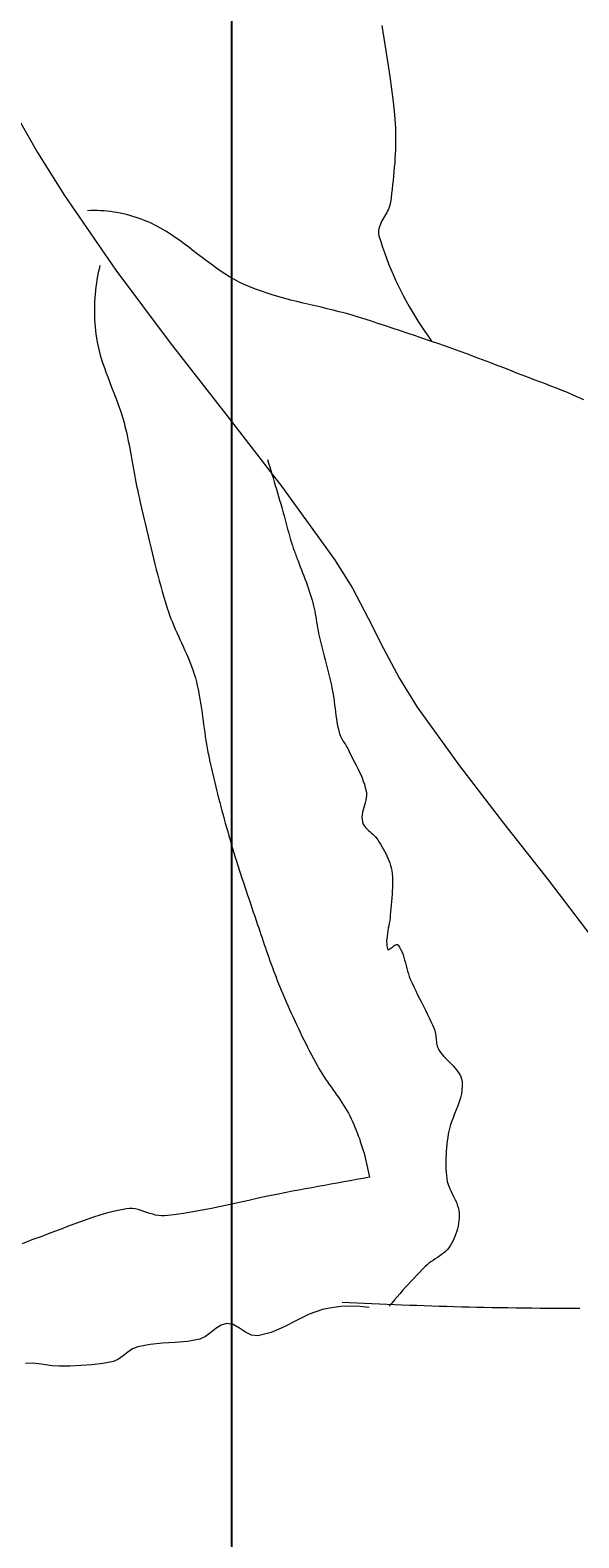
# Model space of a CAD drawing. Units: inches. Extents: x -15 to 423, y -713 to 71.
# Tile 6 of 24: x 57 to 70, y -195 to -159. Entities that reach past the tile are written whole.
import ezdxf

# ---------------------------------------------------------------- set-up
doc = ezdxf.new("R2010")
doc.units = ezdxf.units.IN
doc.header["$MEASUREMENT"] = 0
doc.layers.add('A-ANNO-DIMS', color=2, linetype='Continuous', lineweight=18)
doc.layers.add('A-FURN', color=9, linetype='Continuous', lineweight=13)
doc.styles.get("Standard").update_dxf_attribs({"font": 'arial.ttf'})
doc.dimstyles.get("Standard").update_dxf_attribs({"dimtxt": 0.18, "dimasz": 0.18, "dimexe": 0.18, "dimexo": 0.0625, "dimgap": 0.09, "dimtad": 0, "dimtih": 1, "dimtoh": 1, "dimdec": 0, "dimzin": 0, "dimdsep": 46, "dimlunit": 3, "dimtxsty": 'Standard', "dimcen": 0.09, "dimadec": 0, "dimazin": 0, "dimtfac": 1, "dimtdec": 0, "dimtofl": 0, "dimtmove": 0, "dimatfit": 3, "dimfxl": 1, "dimtolj": 1, "dimtzin": 0, "dimarcsym": 0})

# ---------------------------------------------------------------- blocks, each defined once
blk = doc.blocks.new('*D37')
at = {"layer": 'A-ANNO-DIMS', "color": 0, "lineweight": -2, "transparency": 16777216}
for p, q in [((34.081, -396.437), (34.081, 57.43)), ((34.261, 57.25), (47.648, 57.25)), ((61.698, 57.25), (48.31, 57.25)), ((61.878, -396.437), (61.878, 57.43))]:
    blk.add_line(p, q, dxfattribs=at)
at = {"layer": 'A-ANNO-DIMS', "color": 0, "transparency": 16777216}
for points in [[(34.261, 57.28), (34.261, 57.22), (34.081, 57.25)], [(61.698, 57.28), (61.698, 57.22), (61.878, 57.25)]]:
    blk.add_solid(points, dxfattribs=at)
at = {"layer": 'Defpoints', "color": 0, "transparency": 16777216}
for p in [(61.878, 57.25), (34.081, -396.5), (61.878, -396.5)]:
    blk.add_point(p, dxfattribs=at)
at = {"layer": 'A-ANNO-DIMS', "color": 0, "transparency": 16777216, "insert": (47.979, 57.25), "char_height": 0.18, "attachment_point": 5}
blk.add_mtext('\\A1;2\'-4"', dxfattribs=at)

msp = doc.modelspace()

# ---------------------------------------------------------------- linework, layer by layer
at = {"layer": 'A-FURN'}
for p, q in [((65.39, -159.179), (65.44, -159.477)), ((65.44, -159.477), (65.489, -159.775)), ((65.489, -159.775), (65.536, -160.073)), ((65.536, -160.073), (65.58, -160.372)), ((65.58, -160.372), (65.62, -160.671)), ((65.62, -160.671), (65.657, -160.971)), ((56.745, -161.125), (57.334, -162.155)), ((65.657, -160.971), (65.69, -161.271)), ((65.69, -161.271), (65.699, -161.373)), ((65.699, -161.373), (65.707, -161.474)), ((65.707, -161.474), (65.712, -161.576)), ((65.712, -161.576), (65.715, -161.679)), ((65.715, -161.679), (65.717, -161.781)), ((65.717, -161.781), (65.716, -161.883)), ((57.334, -162.155), (57.961, -163.158)), ((65.707, -162.19), (65.701, -162.292)), ((65.712, -162.088), (65.707, -162.19)), ((65.715, -161.985), (65.712, -162.088)), ((65.716, -161.883), (65.715, -161.985)), ((65.686, -162.497), (65.677, -162.599)), ((65.694, -162.395), (65.686, -162.497)), ((65.701, -162.292), (65.694, -162.395)), ((65.645, -162.905), (65.634, -163.007)), ((65.657, -162.804), (65.645, -162.905)), ((65.667, -162.701), (65.657, -162.804)), ((65.677, -162.599), (65.667, -162.701)), ((57.961, -163.158), (59.163, -164.905)), ((65.609, -163.211), (65.596, -163.312)), ((65.621, -163.109), (65.609, -163.211)), ((65.634, -163.007), (65.621, -163.109)), ((58.581, -163.513), (58.505, -163.516)), ((58.657, -163.512), (58.581, -163.513)), ((58.734, -163.513), (58.657, -163.512)), ((58.81, -163.516), (58.734, -163.513)), ((58.887, -163.52), (58.81, -163.516)), ((58.963, -163.527), (58.887, -163.52)), ((59.04, -163.536), (58.963, -163.527)), ((59.116, -163.546), (59.04, -163.536)), ((59.192, -163.558), (59.116, -163.546)), ((59.268, -163.572), (59.192, -163.558)), ((59.344, -163.588), (59.268, -163.572)), ((59.419, -163.605), (59.344, -163.588)), ((59.493, -163.625), (59.419, -163.605)), ((59.567, -163.646), (59.493, -163.625)), ((65.463, -163.632), (65.44, -163.671)), ((65.485, -163.593), (65.463, -163.632)), ((65.507, -163.554), (65.485, -163.593)), ((65.528, -163.514), (65.507, -163.554)), ((65.547, -163.475), (65.528, -163.514)), ((65.563, -163.434), (65.547, -163.475)), ((65.577, -163.394), (65.563, -163.434)), ((65.588, -163.353), (65.577, -163.394)), ((65.596, -163.312), (65.588, -163.353)), ((59.64, -163.669), (59.567, -163.646)), ((59.713, -163.693), (59.64, -163.669)), ((59.785, -163.72), (59.713, -163.693)), ((59.856, -163.748), (59.785, -163.72)), ((59.926, -163.778), (59.856, -163.748)), ((59.995, -163.809), (59.926, -163.778)), ((60.112, -163.867), (59.995, -163.809)), ((60.226, -163.929), (60.112, -163.867)), ((60.338, -163.995), (60.226, -163.929)), ((65.315, -163.983), (65.314, -164.022)), ((65.321, -163.943), (65.315, -163.983)), ((65.33, -163.904), (65.321, -163.943)), ((65.343, -163.866), (65.33, -163.904)), ((65.359, -163.827), (65.343, -163.866)), ((65.377, -163.788), (65.359, -163.827)), ((65.397, -163.749), (65.377, -163.788)), ((65.418, -163.71), (65.397, -163.749)), ((65.44, -163.671), (65.418, -163.71)), ((60.447, -164.065), (60.338, -163.995)), ((60.556, -164.138), (60.447, -164.065)), ((60.662, -164.213), (60.556, -164.138)), ((60.768, -164.291), (60.662, -164.213)), ((60.873, -164.369), (60.768, -164.291)), ((65.314, -164.022), (65.318, -164.062)), ((65.318, -164.062), (65.327, -164.101)), ((65.327, -164.101), (65.367, -164.233)), ((65.367, -164.233), (65.41, -164.364)), ((60.977, -164.449), (60.873, -164.369)), ((61.081, -164.529), (60.977, -164.449)), ((61.186, -164.609), (61.081, -164.529)), ((61.29, -164.688), (61.186, -164.609)), ((61.395, -164.766), (61.29, -164.688)), ((65.41, -164.364), (65.455, -164.495)), ((65.455, -164.495), (65.502, -164.625)), ((65.502, -164.625), (65.552, -164.754)), ((58.739, -165.044), (58.724, -165.128)), ((58.755, -164.961), (58.739, -165.044)), ((58.774, -164.878), (58.755, -164.961)), ((58.794, -164.796), (58.774, -164.878)), ((59.163, -164.905), (60.438, -166.601)), ((61.501, -164.843), (61.395, -164.766)), ((61.608, -164.917), (61.501, -164.843)), ((61.717, -164.989), (61.608, -164.917)), ((61.828, -165.057), (61.717, -164.989)), ((65.552, -164.754), (65.605, -164.882)), ((65.605, -164.882), (65.659, -165.01)), ((65.659, -165.01), (65.716, -165.136)), ((58.688, -165.382), (58.68, -165.467)), ((58.698, -165.297), (58.688, -165.382)), ((58.71, -165.212), (58.698, -165.297)), ((58.724, -165.128), (58.71, -165.212)), ((61.94, -165.122), (61.828, -165.057)), ((62.055, -165.183), (61.94, -165.122)), ((62.172, -165.239), (62.055, -165.183)), ((62.305, -165.296), (62.172, -165.239)), ((62.439, -165.349), (62.305, -165.296)), ((62.574, -165.399), (62.439, -165.349)), ((62.711, -165.445), (62.574, -165.399)), ((65.716, -165.136), (65.775, -165.262)), ((65.775, -165.262), (65.836, -165.386)), ((65.836, -165.386), (65.899, -165.51)), ((58.665, -165.723), (58.663, -165.808)), ((58.668, -165.637), (58.665, -165.723)), ((58.673, -165.552), (58.668, -165.637)), ((58.68, -165.467), (58.673, -165.552)), ((62.848, -165.488), (62.711, -165.445)), ((62.987, -165.529), (62.848, -165.488)), ((63.126, -165.568), (62.987, -165.529)), ((63.266, -165.605), (63.126, -165.568)), ((63.407, -165.64), (63.266, -165.605)), ((63.548, -165.674), (63.407, -165.64)), ((63.689, -165.708), (63.548, -165.674)), ((63.83, -165.741), (63.689, -165.708)), ((63.972, -165.774), (63.83, -165.741)), ((65.899, -165.51), (65.964, -165.632)), ((65.964, -165.632), (66.032, -165.754)), ((66.032, -165.754), (66.101, -165.873)), ((58.663, -165.808), (58.663, -165.894)), ((58.663, -165.894), (58.665, -165.979)), ((58.665, -165.979), (58.669, -166.064)), ((58.669, -166.064), (58.674, -166.149)), ((64.113, -165.808), (63.972, -165.774)), ((64.254, -165.842), (64.113, -165.808)), ((64.395, -165.877), (64.254, -165.842)), ((64.535, -165.914), (64.395, -165.877)), ((64.675, -165.952), (64.535, -165.914)), ((64.813, -165.993), (64.675, -165.952)), ((64.951, -166.036), (64.813, -165.993)), ((65.127, -166.093), (64.951, -166.036)), ((65.303, -166.151), (65.127, -166.093)), ((66.101, -165.873), (66.173, -165.992)), ((66.173, -165.992), (66.246, -166.109)), ((58.674, -166.149), (58.681, -166.234)), ((58.681, -166.234), (58.689, -166.319)), ((58.689, -166.319), (58.7, -166.403)), ((58.7, -166.403), (58.711, -166.487)), ((65.479, -166.208), (65.303, -166.151)), ((65.655, -166.266), (65.479, -166.208)), ((65.831, -166.325), (65.655, -166.266)), ((66.007, -166.383), (65.831, -166.325)), ((66.182, -166.442), (66.007, -166.383)), ((66.357, -166.502), (66.182, -166.442)), ((66.246, -166.109), (66.322, -166.225)), ((66.322, -166.225), (66.4, -166.339)), ((66.4, -166.339), (66.479, -166.452)), ((66.479, -166.452), (66.56, -166.563)), ((58.711, -166.487), (58.729, -166.589)), ((58.729, -166.589), (58.75, -166.691)), ((58.75, -166.691), (58.775, -166.792)), ((58.775, -166.792), (58.802, -166.892)), ((60.438, -166.601), (61.744, -168.275)), ((66.532, -166.562), (66.357, -166.502)), ((66.707, -166.623), (66.532, -166.562)), ((66.882, -166.684), (66.707, -166.623)), ((67.057, -166.746), (66.882, -166.684)), ((67.231, -166.809), (67.057, -166.746)), ((67.405, -166.872), (67.231, -166.809)), ((58.802, -166.892), (58.832, -166.992)), ((58.832, -166.992), (58.863, -167.091)), ((58.863, -167.091), (58.897, -167.19)), ((67.578, -166.936), (67.405, -166.872)), ((67.752, -167.001), (67.578, -166.936)), ((67.925, -167.067), (67.752, -167.001)), ((68.097, -167.133), (67.925, -167.067)), ((68.27, -167.201), (68.097, -167.133)), ((58.897, -167.19), (58.932, -167.288)), ((58.932, -167.288), (58.969, -167.386)), ((58.969, -167.386), (59.006, -167.484)), ((59.006, -167.484), (59.044, -167.581)), ((68.442, -167.269), (68.27, -167.201)), ((68.57, -167.32), (68.442, -167.269)), ((68.7, -167.37), (68.57, -167.32)), ((68.83, -167.419), (68.7, -167.37)), ((68.961, -167.468), (68.83, -167.419)), ((69.092, -167.517), (68.961, -167.468)), ((69.222, -167.566), (69.092, -167.517)), ((59.044, -167.581), (59.082, -167.679)), ((59.082, -167.679), (59.121, -167.777)), ((59.121, -167.777), (59.158, -167.875)), ((69.353, -167.615), (69.222, -167.566)), ((69.484, -167.666), (69.353, -167.615)), ((69.613, -167.717), (69.484, -167.666)), ((69.742, -167.77), (69.613, -167.717)), ((69.87, -167.825), (69.742, -167.77)), ((69.997, -167.881), (69.87, -167.825)), ((59.158, -167.875), (59.195, -167.973)), ((59.195, -167.973), (59.231, -168.071)), ((59.231, -168.071), (59.265, -168.17)), ((59.265, -168.17), (59.298, -168.269)), ((70.122, -167.94), (69.997, -167.881)), ((59.298, -168.269), (59.329, -168.369)), ((59.329, -168.369), (59.357, -168.469)), ((59.357, -168.469), (59.379, -168.555)), ((59.379, -168.555), (59.4, -168.641)), ((61.744, -168.275), (63.041, -169.957)), ((59.4, -168.641), (59.42, -168.728)), ((59.42, -168.728), (59.439, -168.814)), ((59.439, -168.814), (59.458, -168.901)), ((59.458, -168.901), (59.475, -168.989)), ((59.475, -168.989), (59.492, -169.076)), ((59.492, -169.076), (59.508, -169.163)), ((59.508, -169.163), (59.524, -169.251)), ((59.524, -169.251), (59.54, -169.338)), ((59.54, -169.338), (59.555, -169.426)), ((59.555, -169.426), (59.571, -169.513)), ((59.571, -169.513), (59.586, -169.601)), ((59.586, -169.601), (59.602, -169.688)), ((62.715, -169.335), (62.741, -169.421)), ((62.741, -169.421), (62.768, -169.507)), ((62.768, -169.507), (62.794, -169.594)), ((62.794, -169.594), (62.82, -169.68)), ((59.602, -169.688), (59.618, -169.776)), ((59.618, -169.776), (59.635, -169.863)), ((59.635, -169.863), (59.652, -169.95)), ((59.652, -169.95), (59.67, -170.038)), ((62.82, -169.68), (62.846, -169.766)), ((62.846, -169.766), (62.872, -169.853)), ((62.872, -169.853), (62.898, -169.939)), ((62.898, -169.939), (62.924, -170.026)), ((63.041, -169.957), (64.285, -171.675)), ((59.67, -170.038), (59.689, -170.124)), ((59.689, -170.124), (59.708, -170.211)), ((59.708, -170.211), (59.739, -170.342)), ((62.924, -170.026), (62.95, -170.112)), ((62.95, -170.112), (62.975, -170.199)), ((62.975, -170.199), (63.001, -170.286)), ((63.001, -170.286), (63.026, -170.372)), ((59.739, -170.342), (59.769, -170.472)), ((59.769, -170.472), (59.799, -170.603)), ((59.799, -170.603), (59.83, -170.734)), ((63.026, -170.372), (63.051, -170.459)), ((63.051, -170.459), (63.069, -170.522)), ((63.069, -170.522), (63.086, -170.585)), ((63.086, -170.585), (63.104, -170.648)), ((63.104, -170.648), (63.121, -170.711)), ((59.83, -170.734), (59.86, -170.865)), ((59.86, -170.865), (59.89, -170.995)), ((59.89, -170.995), (59.921, -171.126)), ((63.121, -170.711), (63.137, -170.774)), ((63.137, -170.774), (63.154, -170.837)), ((63.154, -170.837), (63.171, -170.9)), ((63.171, -170.9), (63.188, -170.963)), ((63.188, -170.963), (63.205, -171.026)), ((63.205, -171.026), (63.222, -171.089)), ((59.921, -171.126), (59.952, -171.256)), ((59.952, -171.256), (59.983, -171.387)), ((59.983, -171.387), (60.015, -171.517)), ((63.222, -171.089), (63.24, -171.152)), ((63.24, -171.152), (63.258, -171.215)), ((63.258, -171.215), (63.277, -171.278)), ((63.277, -171.278), (63.287, -171.311)), ((63.287, -171.311), (63.298, -171.344)), ((63.298, -171.344), (63.31, -171.377)), ((63.31, -171.377), (63.321, -171.41)), ((60.015, -171.517), (60.047, -171.648)), ((60.047, -171.648), (60.08, -171.778)), ((63.321, -171.41), (63.333, -171.443)), ((63.333, -171.443), (63.345, -171.476)), ((63.345, -171.476), (63.358, -171.509)), ((63.358, -171.509), (63.37, -171.542)), ((63.37, -171.542), (63.382, -171.575)), ((63.382, -171.575), (63.395, -171.608)), ((63.395, -171.608), (63.407, -171.64)), ((63.407, -171.64), (63.42, -171.673)), ((63.42, -171.673), (63.431, -171.706)), ((63.431, -171.706), (63.457, -171.777)), ((64.285, -171.675), (64.703, -172.347)), ((60.08, -171.778), (60.113, -171.908)), ((60.113, -171.908), (60.147, -172.037)), ((60.147, -172.037), (60.182, -172.167)), ((63.457, -171.777), (63.484, -171.847)), ((63.484, -171.847), (63.511, -171.917)), ((63.511, -171.917), (63.538, -171.988)), ((63.538, -171.988), (63.565, -172.058)), ((63.565, -172.058), (63.592, -172.128)), ((60.182, -172.167), (60.218, -172.296)), ((60.218, -172.296), (60.254, -172.425)), ((60.254, -172.425), (60.291, -172.554)), ((63.592, -172.128), (63.619, -172.198)), ((63.619, -172.198), (63.645, -172.269)), ((63.645, -172.269), (63.671, -172.339)), ((63.671, -172.339), (63.695, -172.41)), ((63.695, -172.41), (63.719, -172.481)), ((64.703, -172.347), (65.076, -173.047)), ((60.291, -172.554), (60.33, -172.682)), ((60.33, -172.682), (60.369, -172.811)), ((63.719, -172.481), (63.742, -172.553)), ((63.742, -172.553), (63.763, -172.625)), ((63.763, -172.625), (63.78, -172.689)), ((63.78, -172.689), (63.795, -172.753)), ((63.795, -172.753), (63.809, -172.817)), ((60.369, -172.811), (60.396, -172.894)), ((60.396, -172.894), (60.425, -172.977)), ((60.425, -172.977), (60.457, -173.059)), ((60.457, -173.059), (60.489, -173.141)), ((60.489, -173.141), (60.523, -173.222)), ((63.809, -172.817), (63.822, -172.882)), ((63.822, -172.882), (63.834, -172.946)), ((63.834, -172.946), (63.845, -173.011)), ((63.845, -173.011), (63.856, -173.076)), ((63.856, -173.076), (63.867, -173.141)), ((63.867, -173.141), (63.878, -173.207)), ((65.076, -173.047), (65.434, -173.756)), ((60.523, -173.222), (60.558, -173.303)), ((60.558, -173.303), (60.594, -173.384)), ((60.594, -173.384), (60.63, -173.464)), ((60.63, -173.464), (60.667, -173.545)), ((63.878, -173.207), (63.889, -173.272)), ((63.889, -173.272), (63.901, -173.336)), ((63.901, -173.336), (63.914, -173.401)), ((63.914, -173.401), (63.927, -173.465)), ((63.927, -173.465), (63.949, -173.559)), ((60.667, -173.545), (60.704, -173.625)), ((60.704, -173.625), (60.741, -173.705)), ((60.741, -173.705), (60.777, -173.785)), ((60.777, -173.785), (60.813, -173.866)), ((60.813, -173.866), (60.848, -173.947)), ((63.949, -173.559), (63.971, -173.652)), ((63.971, -173.652), (63.995, -173.745)), ((63.995, -173.745), (64.018, -173.837)), ((64.018, -173.837), (64.042, -173.93)), ((65.434, -173.756), (65.807, -174.456)), ((60.848, -173.947), (60.882, -174.028)), ((60.882, -174.028), (60.914, -174.11)), ((60.914, -174.11), (60.945, -174.192)), ((60.945, -174.192), (60.974, -174.275)), ((64.042, -173.93), (64.067, -174.023)), ((64.067, -174.023), (64.091, -174.115)), ((64.091, -174.115), (64.115, -174.208)), ((64.115, -174.208), (64.138, -174.301)), ((60.974, -174.275), (61.002, -174.358)), ((61.002, -174.358), (61.027, -174.442)), ((61.027, -174.442), (61.051, -174.532)), ((61.051, -174.532), (61.072, -174.622)), ((64.138, -174.301), (64.161, -174.393)), ((64.161, -174.393), (64.183, -174.487)), ((64.183, -174.487), (64.205, -174.58)), ((65.807, -174.456), (66.223, -175.129)), ((61.072, -174.622), (61.092, -174.712)), ((61.092, -174.712), (61.111, -174.802)), ((61.111, -174.802), (61.128, -174.893)), ((61.128, -174.893), (61.143, -174.985)), ((64.205, -174.58), (64.225, -174.673)), ((64.225, -174.673), (64.24, -174.753)), ((64.24, -174.753), (64.254, -174.834)), ((64.254, -174.834), (64.266, -174.915)), ((64.266, -174.915), (64.277, -174.996)), ((61.143, -174.985), (61.158, -175.076)), ((61.158, -175.076), (61.171, -175.168)), ((61.171, -175.168), (61.184, -175.26)), ((61.184, -175.26), (61.197, -175.352)), ((64.277, -174.996), (64.287, -175.077)), ((64.287, -175.077), (64.297, -175.158)), ((64.297, -175.158), (64.307, -175.239)), ((64.307, -175.239), (64.318, -175.32)), ((66.223, -175.129), (67.211, -176.499)), ((61.197, -175.352), (61.209, -175.444)), ((61.209, -175.444), (61.221, -175.536)), ((61.221, -175.536), (61.233, -175.628)), ((61.233, -175.628), (61.246, -175.72)), ((64.318, -175.32), (64.33, -175.4)), ((64.33, -175.4), (64.343, -175.481)), ((64.343, -175.481), (64.358, -175.561)), ((64.358, -175.561), (64.375, -175.641)), ((61.246, -175.72), (61.259, -175.811)), ((61.259, -175.811), (61.273, -175.903)), ((61.273, -175.903), (61.287, -175.995)), ((64.375, -175.641), (64.394, -175.72)), ((64.394, -175.72), (64.405, -175.753)), ((64.405, -175.753), (64.417, -175.786)), ((64.417, -175.786), (64.432, -175.818)), ((64.432, -175.818), (64.448, -175.85)), ((64.448, -175.85), (64.465, -175.881)), ((64.465, -175.881), (64.483, -175.911)), ((64.483, -175.911), (64.502, -175.942)), ((64.502, -175.942), (64.522, -175.972)), ((64.522, -175.972), (64.541, -176.002)), ((61.287, -175.995), (61.303, -176.086)), ((61.303, -176.086), (61.32, -176.177)), ((61.32, -176.177), (61.339, -176.268)), ((61.339, -176.268), (61.36, -176.367)), ((64.541, -176.002), (64.559, -176.033)), ((64.559, -176.033), (64.577, -176.063)), ((64.577, -176.063), (64.594, -176.094)), ((64.594, -176.094), (64.61, -176.126)), ((64.61, -176.126), (64.645, -176.199)), ((64.645, -176.199), (64.681, -176.271)), ((64.681, -176.271), (64.718, -176.343)), ((61.36, -176.367), (61.382, -176.466)), ((61.382, -176.466), (61.405, -176.565)), ((61.405, -176.565), (61.427, -176.664)), ((61.427, -176.664), (61.45, -176.762)), ((64.718, -176.343), (64.755, -176.415)), ((64.755, -176.415), (64.792, -176.487)), ((64.792, -176.487), (64.829, -176.559)), ((64.829, -176.559), (64.865, -176.632)), ((64.865, -176.632), (64.899, -176.705)), ((67.211, -176.499), (68.243, -177.837)), ((61.45, -176.762), (61.474, -176.861)), ((61.474, -176.861), (61.498, -176.96)), ((61.498, -176.96), (61.522, -177.058)), ((64.899, -176.705), (64.93, -176.779)), ((64.93, -176.779), (64.959, -176.854)), ((64.959, -176.854), (64.985, -176.929)), ((64.985, -176.929), (65.007, -177.006)), ((65.007, -177.006), (65.025, -177.084)), ((61.522, -177.058), (61.547, -177.156)), ((61.547, -177.156), (61.572, -177.255)), ((61.572, -177.255), (61.597, -177.353)), ((61.597, -177.353), (61.623, -177.451)), ((65.002, -177.362), (64.986, -177.419)), ((65.015, -177.306), (65.002, -177.362)), ((65.025, -177.251), (65.015, -177.306)), ((65.025, -177.084), (65.032, -177.139)), ((65.031, -177.195), (65.025, -177.251)), ((65.032, -177.139), (65.031, -177.195)), ((61.623, -177.451), (61.649, -177.549)), ((61.649, -177.549), (61.675, -177.647)), ((61.675, -177.647), (61.702, -177.745)), ((61.702, -177.745), (61.729, -177.843)), ((64.933, -177.642), (64.929, -177.697)), ((64.929, -177.697), (64.93, -177.753)), ((64.943, -177.586), (64.933, -177.642)), ((64.956, -177.531), (64.943, -177.586)), ((64.97, -177.475), (64.956, -177.531)), ((64.986, -177.419), (64.97, -177.475)), ((61.729, -177.843), (61.756, -177.94)), ((61.756, -177.94), (61.784, -178.038)), ((61.784, -178.038), (61.812, -178.135)), ((64.93, -177.753), (64.939, -177.807)), ((64.939, -177.807), (64.952, -177.847)), ((64.952, -177.847), (64.971, -177.884)), ((64.971, -177.884), (64.994, -177.919)), ((64.994, -177.919), (65.021, -177.951)), ((65.021, -177.951), (65.051, -177.982)), ((65.051, -177.982), (65.083, -178.012)), ((65.083, -178.012), (65.117, -178.042)), ((65.117, -178.042), (65.151, -178.071)), ((65.151, -178.071), (65.185, -178.1)), ((68.243, -177.837), (69.287, -179.166)), ((61.812, -178.135), (61.84, -178.233)), ((61.84, -178.233), (61.869, -178.333)), ((61.869, -178.333), (61.899, -178.433)), ((61.899, -178.433), (61.929, -178.532)), ((65.185, -178.1), (65.217, -178.131)), ((65.217, -178.131), (65.248, -178.162)), ((65.248, -178.162), (65.276, -178.196)), ((65.276, -178.196), (65.3, -178.231)), ((65.3, -178.231), (65.331, -178.283)), ((65.331, -178.283), (65.363, -178.335)), ((65.363, -178.335), (65.394, -178.387)), ((65.394, -178.387), (65.425, -178.44)), ((65.425, -178.44), (65.455, -178.494)), ((61.929, -178.532), (61.96, -178.632)), ((61.96, -178.632), (61.991, -178.732)), ((61.991, -178.732), (62.022, -178.831)), ((65.455, -178.494), (65.484, -178.547)), ((65.484, -178.547), (65.511, -178.602)), ((65.511, -178.602), (65.537, -178.657)), ((65.537, -178.657), (65.56, -178.713)), ((65.56, -178.713), (65.581, -178.769)), ((65.581, -178.769), (65.599, -178.827)), ((62.022, -178.831), (62.054, -178.93)), ((62.054, -178.93), (62.086, -179.029)), ((62.086, -179.029), (62.119, -179.128)), ((62.119, -179.128), (62.151, -179.227)), ((65.599, -178.827), (65.615, -178.885)), ((65.615, -178.885), (65.626, -178.944)), ((65.626, -178.944), (65.637, -179.024)), ((65.637, -179.024), (65.644, -179.104)), ((65.644, -179.104), (65.647, -179.185)), ((62.151, -179.227), (62.184, -179.326)), ((62.184, -179.326), (62.217, -179.425)), ((62.217, -179.425), (62.25, -179.524)), ((65.633, -179.509), (65.626, -179.59)), ((65.639, -179.427), (65.633, -179.509)), ((65.644, -179.346), (65.639, -179.427)), ((65.647, -179.265), (65.644, -179.346)), ((65.647, -179.185), (65.647, -179.265)), ((69.287, -179.166), (70.313, -180.508)), ((62.25, -179.524), (62.284, -179.623)), ((62.284, -179.623), (62.317, -179.722)), ((62.317, -179.722), (62.351, -179.82)), ((62.351, -179.82), (62.384, -179.919)), ((65.602, -179.833), (65.595, -179.914)), ((65.61, -179.752), (65.602, -179.833)), ((65.618, -179.671), (65.61, -179.752)), ((65.626, -179.59), (65.618, -179.671)), ((62.384, -179.919), (62.418, -180.018)), ((62.418, -180.018), (62.452, -180.116)), ((62.452, -180.116), (62.485, -180.215)), ((65.567, -180.177), (65.556, -180.238)), ((65.577, -180.116), (65.567, -180.177)), ((65.585, -180.056), (65.577, -180.116)), ((65.59, -179.995), (65.585, -180.056)), ((65.595, -179.914), (65.59, -179.995)), ((62.485, -180.215), (62.511, -180.292)), ((62.511, -180.292), (62.538, -180.369)), ((62.538, -180.369), (62.564, -180.446)), ((62.564, -180.446), (62.59, -180.523)), ((62.59, -180.523), (62.616, -180.601)), ((65.509, -180.542), (65.506, -180.602)), ((65.515, -180.481), (65.509, -180.542)), ((65.523, -180.421), (65.515, -180.481)), ((65.533, -180.36), (65.523, -180.421)), ((65.545, -180.299), (65.533, -180.36)), ((65.556, -180.238), (65.545, -180.299)), ((62.616, -180.601), (62.642, -180.678)), ((62.642, -180.678), (62.668, -180.755)), ((62.668, -180.755), (62.694, -180.832)), ((62.694, -180.832), (62.721, -180.909)), ((62.721, -180.909), (62.748, -180.986)), ((65.506, -180.602), (65.508, -180.661)), ((65.508, -180.661), (65.514, -180.721)), ((65.514, -180.721), (65.527, -180.779)), ((65.527, -180.779), (65.534, -180.793)), ((65.534, -180.793), (65.546, -180.797)), ((65.546, -180.797), (65.562, -180.793)), ((65.562, -180.793), (65.581, -180.783)), ((65.581, -180.783), (65.603, -180.768)), ((65.603, -180.768), (65.626, -180.75)), ((65.626, -180.75), (65.65, -180.731)), ((65.65, -180.731), (65.674, -180.713)), ((65.674, -180.713), (65.698, -180.697)), ((65.698, -180.697), (65.72, -180.685)), ((65.72, -180.685), (65.74, -180.679)), ((65.74, -180.679), (65.758, -180.68)), ((65.758, -180.68), (65.772, -180.691)), ((65.772, -180.691), (65.808, -180.744)), ((65.808, -180.744), (65.839, -180.801)), ((65.839, -180.801), (65.866, -180.859)), ((65.866, -180.859), (65.89, -180.92)), ((65.89, -180.92), (65.91, -180.981)), ((62.748, -180.986), (62.775, -181.063)), ((62.775, -181.063), (62.802, -181.139)), ((62.802, -181.139), (62.83, -181.216)), ((62.83, -181.216), (62.858, -181.292)), ((65.91, -180.981), (65.928, -181.045)), ((65.928, -181.045), (65.945, -181.109)), ((65.945, -181.109), (65.962, -181.173)), ((65.962, -181.173), (65.978, -181.237)), ((65.978, -181.237), (65.995, -181.301)), ((62.858, -181.292), (62.887, -181.368)), ((62.887, -181.368), (62.916, -181.444)), ((62.916, -181.444), (62.945, -181.52)), ((62.945, -181.52), (62.975, -181.596)), ((62.975, -181.596), (63.006, -181.671)), ((65.995, -181.301), (66.014, -181.364)), ((66.014, -181.364), (66.035, -181.427)), ((66.035, -181.427), (66.059, -181.487)), ((66.059, -181.487), (66.1, -181.579)), ((66.1, -181.579), (66.142, -181.671)), ((63.006, -181.671), (63.037, -181.746)), ((63.037, -181.746), (63.076, -181.836)), ((63.076, -181.836), (63.115, -181.927)), ((63.115, -181.927), (63.154, -182.017)), ((66.142, -181.671), (66.186, -181.761)), ((66.186, -181.761), (66.23, -181.852)), ((66.23, -181.852), (66.276, -181.941)), ((66.276, -181.941), (66.322, -182.031)), ((63.154, -182.017), (63.193, -182.107)), ((63.193, -182.107), (63.233, -182.196)), ((63.233, -182.196), (63.274, -182.286)), ((63.274, -182.286), (63.314, -182.375)), ((66.322, -182.031), (66.367, -182.121)), ((66.367, -182.121), (66.413, -182.211)), ((66.413, -182.211), (66.457, -182.301)), ((66.457, -182.301), (66.501, -182.392)), ((63.314, -182.375), (63.355, -182.464)), ((63.355, -182.464), (63.397, -182.553)), ((63.397, -182.553), (63.439, -182.642)), ((63.439, -182.642), (63.481, -182.731)), ((66.501, -182.392), (66.544, -182.483)), ((66.544, -182.483), (66.584, -182.575)), ((66.584, -182.575), (66.623, -182.668)), ((66.623, -182.668), (66.635, -182.701)), ((63.481, -182.731), (63.524, -182.819)), ((63.524, -182.819), (63.567, -182.907)), ((63.567, -182.907), (63.611, -182.995)), ((63.611, -182.995), (63.655, -183.083)), ((66.635, -182.701), (66.644, -182.736)), ((66.644, -182.736), (66.65, -182.771)), ((66.65, -182.771), (66.655, -182.806)), ((66.655, -182.806), (66.659, -182.842)), ((66.659, -182.842), (66.663, -182.878)), ((66.663, -182.878), (66.666, -182.914)), ((66.666, -182.914), (66.67, -182.95)), ((66.67, -182.95), (66.675, -182.985)), ((66.675, -182.985), (66.681, -183.02)), ((66.681, -183.02), (66.69, -183.054)), ((63.655, -183.083), (63.7, -183.17)), ((63.7, -183.17), (63.745, -183.258)), ((63.745, -183.258), (63.791, -183.344)), ((63.791, -183.344), (63.837, -183.431)), ((66.69, -183.054), (66.702, -183.087)), ((66.702, -183.087), (66.716, -183.119)), ((66.716, -183.119), (66.754, -183.182)), ((66.754, -183.182), (66.798, -183.241)), ((66.798, -183.241), (66.847, -183.299)), ((66.847, -183.299), (66.9, -183.354)), ((66.9, -183.354), (66.954, -183.409)), ((63.837, -183.431), (63.884, -183.517)), ((63.884, -183.517), (63.92, -183.581)), ((63.92, -183.581), (63.957, -183.645)), ((63.957, -183.645), (63.996, -183.707)), ((63.996, -183.707), (64.036, -183.769)), ((66.954, -183.409), (67.008, -183.463)), ((67.008, -183.463), (67.062, -183.518)), ((67.062, -183.518), (67.112, -183.573)), ((67.112, -183.573), (67.158, -183.63)), ((67.158, -183.63), (67.199, -183.69)), ((67.199, -183.69), (67.232, -183.752)), ((64.036, -183.769), (64.077, -183.83)), ((64.077, -183.83), (64.119, -183.89)), ((64.119, -183.89), (64.161, -183.951)), ((64.161, -183.951), (64.204, -184.011)), ((64.204, -184.011), (64.247, -184.071)), ((64.247, -184.071), (64.29, -184.131)), ((67.232, -183.752), (67.256, -183.818)), ((67.256, -183.818), (67.271, -183.888)), ((67.27, -184.079), (67.256, -184.174)), ((67.276, -183.984), (67.27, -184.079)), ((67.271, -183.888), (67.276, -183.984)), ((64.29, -184.131), (64.333, -184.191)), ((64.333, -184.191), (64.375, -184.251)), ((64.375, -184.251), (64.417, -184.312)), ((64.417, -184.312), (64.458, -184.373)), ((64.458, -184.373), (64.498, -184.434)), ((64.498, -184.434), (64.537, -184.497)), ((67.204, -184.361), (67.171, -184.454)), ((67.233, -184.267), (67.204, -184.361)), ((67.256, -184.174), (67.233, -184.267)), ((64.537, -184.497), (64.574, -184.56)), ((64.574, -184.56), (64.61, -184.624)), ((64.61, -184.624), (64.644, -184.689)), ((64.644, -184.689), (64.676, -184.755)), ((64.676, -184.755), (64.706, -184.82)), ((67.061, -184.733), (67.026, -184.827)), ((67.098, -184.64), (67.061, -184.733)), ((67.135, -184.547), (67.098, -184.64)), ((67.171, -184.454), (67.135, -184.547)), ((64.706, -184.82), (64.735, -184.885)), ((64.735, -184.885), (64.763, -184.951)), ((64.763, -184.951), (64.79, -185.018)), ((64.79, -185.018), (64.817, -185.085)), ((64.817, -185.085), (64.842, -185.152)), ((66.95, -185.111), (66.938, -185.191)), ((66.969, -185.015), (66.95, -185.111)), ((66.995, -184.921), (66.969, -185.015)), ((67.026, -184.827), (66.995, -184.921)), ((64.842, -185.152), (64.867, -185.22)), ((64.867, -185.22), (64.89, -185.288)), ((64.89, -185.288), (64.913, -185.356)), ((64.913, -185.356), (64.935, -185.425)), ((64.935, -185.425), (64.956, -185.494)), ((64.956, -185.494), (64.976, -185.563)), ((66.909, -185.433), (66.902, -185.514)), ((66.917, -185.352), (66.909, -185.433)), ((66.927, -185.272), (66.917, -185.352)), ((66.938, -185.191), (66.927, -185.272)), ((64.976, -185.563), (64.995, -185.632)), ((64.995, -185.632), (65.013, -185.702)), ((65.013, -185.702), (65.03, -185.772)), ((65.03, -185.772), (65.046, -185.842)), ((65.046, -185.842), (65.061, -185.912)), ((66.892, -185.677), (66.891, -185.758)), ((66.891, -185.758), (66.891, -185.839)), ((66.891, -185.839), (66.893, -185.92)), ((66.896, -185.596), (66.892, -185.677)), ((66.902, -185.514), (66.896, -185.596)), ((64.651, -186.205), (64.501, -186.232)), ((64.801, -186.178), (64.651, -186.205)), ((64.951, -186.151), (64.801, -186.178)), ((65.101, -186.124), (64.951, -186.151)), ((65.061, -185.912), (65.075, -185.983)), ((65.075, -185.983), (65.088, -186.053)), ((65.088, -186.053), (65.101, -186.124)), ((66.893, -185.92), (66.898, -186.001)), ((66.898, -186.001), (66.905, -186.082)), ((66.905, -186.082), (66.914, -186.162)), ((66.914, -186.162), (66.926, -186.226)), ((62.934, -186.523), (62.715, -186.568)), ((63.153, -186.48), (62.934, -186.523)), ((63.302, -186.452), (63.153, -186.48)), ((63.452, -186.425), (63.302, -186.452)), ((63.602, -186.397), (63.452, -186.425)), ((63.752, -186.369), (63.602, -186.397)), ((63.902, -186.341), (63.752, -186.369)), ((64.051, -186.314), (63.902, -186.341)), ((64.201, -186.286), (64.051, -186.314)), ((64.351, -186.259), (64.201, -186.286)), ((64.501, -186.232), (64.351, -186.259)), ((66.926, -186.226), (66.944, -186.289)), ((66.944, -186.289), (66.967, -186.35)), ((66.967, -186.35), (66.993, -186.41)), ((66.993, -186.41), (67.022, -186.47)), ((67.022, -186.47), (67.051, -186.53)), ((67.051, -186.53), (67.082, -186.589)), ((59.256, -186.889), (59.1, -186.925)), ((59.413, -186.86), (59.256, -186.889)), ((59.482, -186.853), (59.413, -186.86)), ((59.55, -186.856), (59.482, -186.853)), ((59.619, -186.865), (59.55, -186.856)), ((59.687, -186.881), (59.619, -186.865)), ((59.755, -186.9), (59.687, -186.881)), ((59.823, -186.923), (59.755, -186.9)), ((61.185, -186.893), (60.966, -186.932)), ((61.404, -186.85), (61.185, -186.893)), ((61.623, -186.805), (61.404, -186.85)), ((61.841, -186.759), (61.623, -186.805)), ((62.06, -186.711), (61.841, -186.759)), ((62.278, -186.663), (62.06, -186.711)), ((62.496, -186.615), (62.278, -186.663)), ((62.715, -186.568), (62.496, -186.615)), ((67.082, -186.589), (67.111, -186.649)), ((67.111, -186.649), (67.138, -186.709)), ((67.138, -186.709), (67.161, -186.77)), ((67.161, -186.77), (67.18, -186.832)), ((67.18, -186.832), (67.194, -186.894)), ((67.194, -186.894), (67.201, -186.959)), ((58.184, -187.221), (58.033, -187.278)), ((58.335, -187.165), (58.184, -187.221)), ((58.486, -187.111), (58.335, -187.165)), ((58.639, -187.059), (58.486, -187.111)), ((58.791, -187.01), (58.639, -187.059)), ((58.945, -186.965), (58.791, -187.01)), ((59.1, -186.925), (58.945, -186.965)), ((59.891, -186.946), (59.823, -186.923)), ((59.96, -186.969), (59.891, -186.946)), ((60.028, -186.99), (59.96, -186.969)), ((60.097, -187.008), (60.028, -186.99)), ((60.165, -187.02), (60.097, -187.008)), ((60.234, -187.026), (60.165, -187.02)), ((60.303, -187.024), (60.234, -187.026)), ((60.525, -186.998), (60.303, -187.024)), ((60.746, -186.967), (60.525, -186.998)), ((60.966, -186.932), (60.746, -186.967)), ((67.177, -187.266), (67.163, -187.327)), ((67.188, -187.205), (67.177, -187.266)), ((67.196, -187.143), (67.188, -187.205)), ((67.201, -187.081), (67.196, -187.143)), ((67.201, -186.959), (67.203, -187.02)), ((67.203, -187.02), (67.201, -187.081)), ((57.201, -187.59), (56.972, -187.679)), ((57.431, -187.505), (57.201, -187.59)), ((57.582, -187.45), (57.431, -187.505)), ((57.733, -187.393), (57.582, -187.45)), ((57.883, -187.336), (57.733, -187.393)), ((58.033, -187.278), (57.883, -187.336)), ((67.054, -187.619), (67.025, -187.673)), ((67.081, -187.563), (67.054, -187.619)), ((67.106, -187.505), (67.081, -187.563)), ((67.127, -187.447), (67.106, -187.505)), ((67.147, -187.387), (67.127, -187.447)), ((67.163, -187.327), (67.147, -187.387)), ((66.742, -187.966), (66.693, -188)), ((66.79, -187.932), (66.742, -187.966)), ((66.837, -187.896), (66.79, -187.932)), ((66.881, -187.858), (66.837, -187.896)), ((66.922, -187.817), (66.881, -187.858)), ((66.96, -187.773), (66.922, -187.817)), ((66.993, -187.726), (66.96, -187.773)), ((67.025, -187.673), (66.993, -187.726)), ((66.34, -188.282), (66.272, -188.35)), ((66.408, -188.214), (66.34, -188.282)), ((66.451, -188.174), (66.408, -188.214)), ((66.497, -188.136), (66.451, -188.174)), ((66.544, -188.101), (66.497, -188.136)), ((66.593, -188.067), (66.544, -188.101)), ((66.643, -188.033), (66.593, -188.067)), ((66.693, -188), (66.643, -188.033)), ((66.007, -188.63), (65.942, -188.702)), ((66.073, -188.56), (66.007, -188.63)), ((66.139, -188.489), (66.073, -188.56)), ((66.205, -188.42), (66.139, -188.489)), ((66.272, -188.35), (66.205, -188.42)), ((65.689, -188.992), (65.627, -189.066)), ((65.751, -188.919), (65.689, -188.992)), ((65.814, -188.846), (65.751, -188.919)), ((65.878, -188.774), (65.814, -188.846)), ((65.942, -188.702), (65.878, -188.774)), ((63.695, -189.327), (63.398, -189.471)), ((64.002, -189.22), (63.695, -189.327)), ((64.216, -189.175), (64.002, -189.22)), ((64.435, -189.147), (64.216, -189.175)), ((64.655, -189.138), (64.435, -189.147)), ((64.637, -189.062), (64.461, -189.054)), ((64.812, -189.07), (64.637, -189.062)), ((64.875, -189.146), (64.655, -189.138)), ((64.987, -189.078), (64.812, -189.07)), ((65.093, -189.173), (64.875, -189.146)), ((65.162, -189.086), (64.987, -189.078)), ((65.337, -189.093), (65.162, -189.086)), ((65.512, -189.1), (65.337, -189.093)), ((65.688, -189.107), (65.512, -189.1)), ((65.627, -189.066), (65.565, -189.14)), ((65.863, -189.113), (65.688, -189.107)), ((66.038, -189.12), (65.863, -189.113)), ((66.213, -189.126), (66.038, -189.12)), ((66.388, -189.132), (66.213, -189.126)), ((66.564, -189.138), (66.388, -189.132)), ((66.739, -189.143), (66.564, -189.138)), ((66.914, -189.148), (66.739, -189.143)), ((67.089, -189.153), (66.914, -189.148)), ((67.265, -189.158), (67.089, -189.153)), ((67.44, -189.162), (67.265, -189.158)), ((67.615, -189.167), (67.44, -189.162)), ((67.79, -189.171), (67.615, -189.167)), ((67.966, -189.175), (67.79, -189.171)), ((68.153, -189.178), (67.966, -189.175)), ((68.341, -189.181), (68.153, -189.178)), ((68.528, -189.184), (68.341, -189.181)), ((68.716, -189.186), (68.528, -189.184)), ((68.903, -189.188), (68.716, -189.186)), ((69.09, -189.189), (68.903, -189.188)), ((69.278, -189.19), (69.09, -189.189)), ((69.465, -189.191), (69.278, -189.19)), ((69.653, -189.191), (69.465, -189.191)), ((69.84, -189.192), (69.653, -189.191)), ((70.028, -189.192), (69.84, -189.192)), ((61.506, -189.659), (61.389, -189.756)), ((61.629, -189.579), (61.506, -189.659)), ((61.765, -189.542), (61.629, -189.579)), ((61.916, -189.57), (61.765, -189.542)), ((62.059, -189.649), (61.916, -189.57)), ((62.2, -189.743), (62.059, -189.649)), ((63.105, -189.622), (62.806, -189.752)), ((63.398, -189.471), (63.105, -189.622)), ((59.677, -190.087), (59.557, -190.139)), ((59.966, -190.033), (59.677, -190.087)), ((60.259, -190.007), (59.966, -190.033)), ((60.554, -189.989), (60.259, -190.007)), ((60.847, -189.962), (60.554, -189.989)), ((61.135, -189.907), (60.847, -189.962)), ((61.268, -189.847), (61.135, -189.907)), ((61.389, -189.756), (61.268, -189.847)), ((62.343, -189.816), (62.2, -189.743)), ((62.493, -189.833), (62.343, -189.816)), ((62.806, -189.752), (62.493, -189.833)), ((59.109, -190.43), (58.859, -190.481)), ((59.23, -190.379), (59.109, -190.43)), ((59.34, -190.302), (59.23, -190.379)), ((59.447, -190.216), (59.34, -190.302)), ((59.557, -190.139), (59.447, -190.216)), ((57.206, -190.469), (57.051, -190.481)), ((57.363, -190.484), (57.206, -190.469)), ((57.52, -190.51), (57.363, -190.484)), ((57.677, -190.535), (57.52, -190.51)), ((57.835, -190.544), (57.677, -190.535)), ((58.091, -190.538), (57.835, -190.544)), ((58.348, -190.529), (58.091, -190.538)), ((58.605, -190.512), (58.348, -190.529)), ((58.859, -190.481), (58.605, -190.512))]:
    msp.add_line(p, q, dxfattribs=at)

# ---------------------------------------------------------------- dimensions: what is measured, and where the dimension line sits
at = {"layer": 'A-ANNO-DIMS'}
dim = msp.add_linear_dim(base=(61.878, 57.25), p1=(34.081, -396.5), p2=(61.878, -396.5), dimstyle='Standard', override={"dimdec": 1, "dimlfac": 1, "dimrnd": 0, "dimzin": 1, "dimdsep": 46, "dimlunit": 4, "dimfrac": 2}, dxfattribs=at)
dim.commit()
dim.dimension.update_dxf_attribs({"geometry": '*D37', "text_midpoint": (47.979, 57.25)})

doc.saveas('drawing.dxf')
